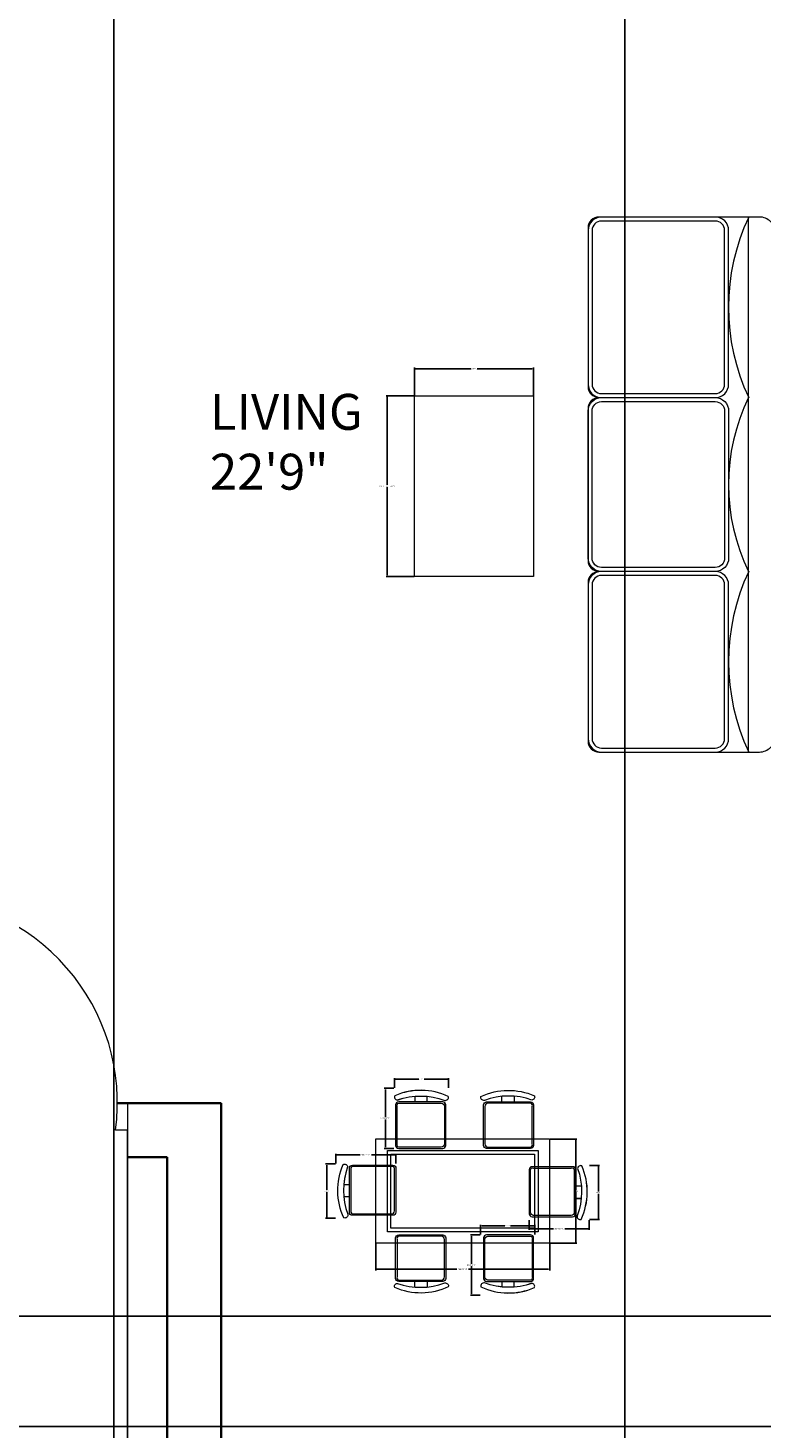
# Model space of a CAD drawing. Units: inches. Extents: x 1854 to 2495, y 1460 to 2772.
# Tile 9 of 12: x 2117 to 2239, y 1958 to 2192. Entities that reach past the tile are written whole.
import ezdxf

# ---------------------------------------------------------------- set-up
doc = ezdxf.new("R2010")
doc.units = ezdxf.units.IN
for name, color, linetype, lineweight in [('A-ANNO-DIMS', 2, 'Continuous', 18), ('A-AREA-IDEN', 7, 'Continuous', 18), ('A-DOOR', 3, 'Continuous', 18), ('A-FURN', 8, 'Continuous', 13), ('A-WALL', 7, 'Continuous', 35)]:
    doc.layers.add(name, color=color, linetype=linetype, lineweight=lineweight)
doc.styles.get("Standard").update_dxf_attribs({"font": 'arial.ttf'})
doc.dimstyles.get("Standard").update_dxf_attribs({"dimtxt": 0.18, "dimasz": 0.18, "dimexe": 0.18, "dimexo": 0.0625, "dimgap": 0.09, "dimtad": 0, "dimtih": 1, "dimtoh": 1, "dimdec": 4, "dimzin": 0, "dimdsep": 46, "dimtxsty": 'Standard', "dimcen": 0.09, "dimadec": 0, "dimazin": 0, "dimtfac": 1, "dimtdec": 4, "dimtofl": 0, "dimtmove": 0, "dimatfit": 3, "dimfxl": 1, "dimtolj": 1, "dimtzin": 0, "dimarcsym": 0})

# ---------------------------------------------------------------- blocks, each defined once
blk = doc.blocks.new('TABLE-COFFEE')
blk.add_lwpolyline([(0, 30.16), (19.85, 30.16), (19.85, 0), (0, 0)], close=True)
blk = doc.blocks.new('DINING-TABLE')
for points in [[(0, 17.41), (29.01, 17.41), (29.01, 0), (0, 0)], [(0, 17.41), (29.01, 17.41), (29.01, 0), (0, 0)], [(1.93, 15.47), (27.08, 15.47), (27.08, 1.93), (1.93, 1.93)], [(1.93, 15.47), (27.08, 15.47), (27.08, 1.93), (1.93, 1.93)], [(2.51, 14.89), (26.5, 14.89), (26.5, 2.51), (2.51, 2.51)], [(2.51, 14.89), (26.5, 14.89), (26.5, 2.51), (2.51, 2.51)]]:
    blk.add_lwpolyline(points, close=True)
blk = doc.blocks.new('DINING-CHAIR-END')
for points in [[(1.68, 0.62, -0.578392), (1.02, 0.02, -0.214524), (0.9, 8.94, -0.552014), (1.62, 8.53, 0.175809), (1.68, 0.62)], [(1.68, 0.62, -0.578392), (1.02, 0.02, -0.214524), (0.9, 8.94, -0.552014), (1.62, 8.52, 0.175809), (1.68, 0.62)], [(1.93, 8.29, -0.414214), (2.45, 8.81), (9.19, 8.81, -0.414214), (9.7, 8.29), (9.7, 0.96, -0.414214), (9.19, 0.45), (2.45, 0.45, -0.414214), (1.93, 0.96), (1.93, 8.29)], [(1.93, 8.29, -0.414214), (2.45, 8.81), (9.19, 8.81, -0.414214), (9.7, 8.29), (9.7, 0.96, -0.414214), (9.19, 0.45), (2.45, 0.45, -0.414214), (1.93, 0.96), (1.93, 8.29)], [(1.93, 3.54), (1, 3.54, 0.064759)], [(1.93, 3.54), (1, 3.54, 0.064759)]]:
    blk.add_lwpolyline(points, format="xyb")
blk.add_lwpolyline([(2.16, 8.29), (2.16, 1.19, 0.414214), (2.68, 0.68), (8.96, 0.68, 0.414214), (9.47, 1.19), (9.47, 8.29, 0.512069), (8.96, 8.58), (2.68, 8.58, 0.512069)], format="xyb", close=True)
blk.add_lwpolyline([(2.16, 8.29), (2.16, 1.19, 0.414214), (2.68, 0.68), (8.96, 0.68, 0.414214), (9.47, 1.19), (9.47, 8.29, 0.512069), (8.96, 8.58), (2.68, 8.58, 0.512069)], format="xyb", close=True)
blk.add_lwpolyline([(0.99, 5.59), (1.93, 5.59)])
blk.add_lwpolyline([(0.99, 5.59), (1.93, 5.59)])
blk = doc.blocks.new('DINING-CHAIR-01')
for points in [[(0.47, 8.09, -0.175809), (8.38, 8.03, 0.578392), (8.98, 8.69, 0.214524), (0.06, 8.81, 0.552014), (0.47, 8.09, -0.065079)], [(8.04, 7.77), (0.71, 7.77, 0.414214), (0.19, 7.26), (0.19, 0.51, 0.414214), (0.71, 0), (8.04, 0, 0.414214), (8.55, 0.51), (8.55, 7.26, 0.414214), (8.04, 7.77)], [(5.46, 7.77), (5.46, 8.7, -0.064759)]]:
    blk.add_lwpolyline(points, format="xyb")
blk.add_lwpolyline([(0.71, 7.54), (7.81, 7.54, -0.414214), (8.32, 7.03), (8.32, 0.74, -0.414214), (7.81, 0.23), (0.71, 0.23, -0.512069), (0.42, 0.74), (0.42, 7.03, -0.512069)], format="xyb", close=True)
blk.add_lwpolyline([(3.41, 8.72), (3.41, 7.77)])
blk = doc.blocks.new('DINING-CHAIR-04')
for points in [[(7.77, 8.29, 0.414214), (7.26, 8.81), (0.51, 8.81, 0.414214), (0, 8.29), (0, 0.96, 0.414214), (0.51, 0.44), (7.26, 0.44, 0.414214), (7.77, 0.96), (7.77, 8.29)], [(8.09, 8.52, -0.175809), (8.03, 0.62, 0.578392), (8.69, 0.02, 0.214524), (8.81, 8.94, 0.552014), (8.09, 8.52, -0.065079)], [(7.77, 3.53), (8.7, 3.53, -0.064759)]]:
    blk.add_lwpolyline(points, format="xyb")
blk.add_lwpolyline([(7.54, 8.29), (7.54, 1.19, -0.414214), (7.03, 0.68), (0.74, 0.68, -0.414214), (0.23, 1.19), (0.23, 8.29, -0.512069), (0.74, 8.58), (7.03, 8.58, -0.512069)], format="xyb", close=True)
blk.add_lwpolyline([(8.72, 5.59), (7.77, 5.59)])
blk = doc.blocks.new('DINING-CHAIR-06')
for points in [[(8.29, 1.93, 0.414214), (8.81, 2.45), (8.81, 9.19, 0.414214), (8.29, 9.7), (0.96, 9.7, 0.414214), (0.44, 9.19), (0.44, 2.45, 0.414214), (0.96, 1.93), (8.29, 1.93)], [(8.52, 1.62, -0.175809), (0.62, 1.68, 0.578392), (0.02, 1.02, 0.214524), (8.94, 0.9, 0.552014), (8.52, 1.62, -0.065079)], [(3.53, 1.93), (3.53, 1, -0.064759)]]:
    blk.add_lwpolyline(points, format="xyb")
blk.add_lwpolyline([(8.29, 2.16), (1.19, 2.16, -0.414214), (0.68, 2.68), (0.68, 8.96, -0.414214), (1.19, 9.47), (8.29, 9.47, -0.512069), (8.58, 8.96), (8.58, 2.68, -0.512069)], format="xyb", close=True)
blk.add_lwpolyline([(5.59, 0.99), (5.59, 1.93)])
blk = doc.blocks.new('SOFA-3-SEAT')
for points in [[(2.23, 59.19), (21.22, 59.19, 0.414214), (23.45, 61.43), (23.45, 87.12, 0.414214), (21.22, 89.35), (2.23, 89.35, 0.414214), (0, 87.12), (0, 61.43, 0.414214)], [(2.23, 59.19), (21.22, 59.19, -0.414214), (23.45, 56.96), (23.45, 32.39, -0.414214), (21.22, 30.16), (2.23, 30.16, -0.414214), (0, 32.39), (0, 56.96, -0.414214)], [(2.23, 0), (21.22, 0, 0.414214), (23.45, 2.23), (23.45, 27.92, 0.414214), (21.22, 30.16), (2.23, 30.16, 0.414214), (0, 27.92), (0, 2.23, 0.414214)]]:
    blk.add_lwpolyline(points, format="xyb", close=True)
at = {"ltscale": 0.03}
blk.add_lwpolyline([(0, 28.35), (0, 1.79, 0.414214), (1.79, 0), (28.59, 0, 0.414214), (31.27, 2.68), (31.27, 86.67, 0.414214), (28.59, 89.35), (1.79, 89.35, 0.414214), (0, 87.56), (0, 61, 0.414214), (1.79, 59.22, -1), (1.79, 59.17, 0.414214), (0, 57.38), (0, 31.96, 0.414214), (1.79, 30.18, -1), (1.79, 30.13, 0.414214)], format="xyb", close=True, dxfattribs=at)
blk.add_lwpolyline([(26.8, 0), (26.8, 89.35)])
for centre, radius, start, end in [((58.64, 74.27), 35.22, 154.6538, 205.3462), ((56.4, 44.67), 32.97, 153.869, 206.131), ((59.01, 15.08), 35.56, 154.9106, 205.0894)]:
    blk.add_arc(centre, radius, start, end)
blk = doc.blocks.new('*D23')
at = {"layer": 'A-ANNO-DIMS', "color": 0, "lineweight": -2, "transparency": 16777216}
for p, q in [((2181.17, 2130.19), (2176.52, 2130.19)), ((2176.7, 2130.01), (2176.7, 2115.3)), ((2176.7, 2100.21), (2176.7, 2114.93)), ((2181.17, 2100.03), (2176.52, 2100.03))]:
    blk.add_line(p, q, dxfattribs=at)
at = {"layer": 'A-ANNO-DIMS', "color": 0, "transparency": 16777216}
for points in [[(2176.67, 2130.01), (2176.73, 2130.01), (2176.7, 2130.19)], [(2176.67, 2100.21), (2176.73, 2100.21), (2176.7, 2100.03)]]:
    blk.add_solid(points, dxfattribs=at)
at = {"layer": 'Defpoints', "color": 0, "transparency": 16777216}
for p in [(2176.7, 2130.19), (2181.23, 2130.19), (2181.23, 2100.03)]:
    blk.add_point(p, dxfattribs=at)
at = {"layer": 'A-ANNO-DIMS', "color": 0, "transparency": 16777216, "insert": (2176.7, 2115.11), "char_height": 0.18, "attachment_point": 5}
blk.add_mtext('\\A1;COFFEE TABLE 30 TYP.', dxfattribs=at)
blk = doc.blocks.new('*D24')
at = {"layer": 'A-ANNO-DIMS', "color": 0, "lineweight": -2, "transparency": 16777216}
for p, q in [((2181.23, 2130.26), (2181.23, 2134.9)), ((2181.41, 2134.72), (2190.62, 2134.72)), ((2200.9, 2134.72), (2191.68, 2134.72)), ((2201.08, 2130.26), (2201.08, 2134.9))]:
    blk.add_line(p, q, dxfattribs=at)
at = {"layer": 'A-ANNO-DIMS', "color": 0, "transparency": 16777216}
for points in [[(2181.41, 2134.75), (2181.41, 2134.69), (2181.23, 2134.72)], [(2200.9, 2134.75), (2200.9, 2134.69), (2201.08, 2134.72)]]:
    blk.add_solid(points, dxfattribs=at)
at = {"layer": 'Defpoints', "color": 0, "transparency": 16777216}
for p in [(2201.08, 2134.72), (2181.23, 2130.19), (2201.08, 2130.19)]:
    blk.add_point(p, dxfattribs=at)
at = {"layer": 'A-ANNO-DIMS', "color": 0, "transparency": 16777216, "insert": (2191.15, 2134.72), "char_height": 0.18, "attachment_point": 5}
blk.add_mtext('\\A1;20 TYP.', dxfattribs=at)
blk = doc.blocks.new('*D33')
at = {"layer": 'A-ANNO-DIMS', "color": 0, "lineweight": -2, "transparency": 16777216}
for p, q in [((2174.78, 1988.6), (2174.78, 1984.13)), ((2203.8, 1988.6), (2203.8, 1984.13)), ((2174.96, 1984.31), (2188.33, 1984.31)), ((2203.62, 1984.31), (2190.25, 1984.31))]:
    blk.add_line(p, q, dxfattribs=at)
at = {"layer": 'A-ANNO-DIMS', "color": 0, "transparency": 16777216}
for points in [[(2174.96, 1984.34), (2174.96, 1984.28), (2174.78, 1984.31)], [(2203.62, 1984.34), (2203.62, 1984.28), (2203.8, 1984.31)]]:
    blk.add_solid(points, dxfattribs=at)
at = {"layer": 'Defpoints', "color": 0, "transparency": 16777216}
for p in [(2174.78, 1988.66), (2203.8, 1988.66), (2203.8, 1984.31)]:
    blk.add_point(p, dxfattribs=at)
at = {"layer": 'A-ANNO-DIMS', "color": 0, "transparency": 16777216, "insert": (2189.29, 1984.31), "char_height": 0.18, "attachment_point": 5}
blk.add_mtext('\\A1;TABLE 29 TYP.', dxfattribs=at)
blk = doc.blocks.new('*D34')
at = {"layer": 'A-ANNO-DIMS', "color": 0, "lineweight": -2, "transparency": 16777216}
for p, q in [((2203.86, 2006.07), (2208.33, 2006.07)), ((2208.15, 2005.89), (2208.15, 1997.55)), ((2208.15, 1988.84), (2208.15, 1997.19)), ((2203.86, 1988.66), (2208.33, 1988.66))]:
    blk.add_line(p, q, dxfattribs=at)
at = {"layer": 'A-ANNO-DIMS', "color": 0, "transparency": 16777216}
for points in [[(2208.12, 2005.89), (2208.18, 2005.89), (2208.15, 2006.07)], [(2208.12, 1988.84), (2208.18, 1988.84), (2208.15, 1988.66)]]:
    blk.add_solid(points, dxfattribs=at)
at = {"layer": 'Defpoints', "color": 0, "transparency": 16777216}
for p in [(2203.8, 2006.07), (2208.15, 2006.07), (2203.8, 1988.66)]:
    blk.add_point(p, dxfattribs=at)
at = {"layer": 'A-ANNO-DIMS', "color": 0, "transparency": 16777216, "insert": (2208.15, 1997.37), "char_height": 0.18, "attachment_point": 5}
blk.add_mtext('\\A1;17 TYP.', dxfattribs=at)
blk = doc.blocks.new('*D39')
at = {"layer": 'A-ANNO-DIMS', "color": 0, "lineweight": -2, "transparency": 16777216}
for p, q in [((2168.09, 2001.96), (2168.09, 2003.59)), ((2168.27, 2003.41), (2172.17, 2003.41)), ((2177.95, 2003.41), (2174.06, 2003.41)), ((2178.13, 2001.96), (2178.13, 2003.59))]:
    blk.add_line(p, q, dxfattribs=at)
at = {"layer": 'A-ANNO-DIMS', "color": 0, "transparency": 16777216}
for points in [[(2168.27, 2003.44), (2168.27, 2003.38), (2168.09, 2003.41)], [(2177.95, 2003.44), (2177.95, 2003.38), (2178.13, 2003.41)]]:
    blk.add_solid(points, dxfattribs=at)
at = {"layer": 'Defpoints', "color": 0, "transparency": 16777216}
for p in [(2168.09, 2001.9), (2178.13, 2003.41), (2178.13, 2001.9)]:
    blk.add_point(p, dxfattribs=at)
at = {"layer": 'A-ANNO-DIMS', "color": 0, "transparency": 16777216, "insert": (2173.11, 2003.41), "char_height": 0.18, "attachment_point": 5}
blk.add_mtext('\\A1;END A 10 TYP.', dxfattribs=at)
blk = doc.blocks.new('*D40')
at = {"layer": 'A-ANNO-DIMS', "color": 0, "lineweight": -2, "transparency": 16777216}
for p, q in [((2168.03, 2001.9), (2166.4, 2001.9)), ((2166.58, 2001.72), (2166.58, 1997.56)), ((2166.58, 1993.03), (2166.58, 1997.19)), ((2168.03, 1992.85), (2166.4, 1992.85))]:
    blk.add_line(p, q, dxfattribs=at)
at = {"layer": 'A-ANNO-DIMS', "color": 0, "transparency": 16777216}
for points in [[(2166.55, 2001.72), (2166.61, 2001.72), (2166.58, 2001.9)], [(2166.55, 1993.03), (2166.61, 1993.03), (2166.58, 1992.85)]]:
    blk.add_solid(points, dxfattribs=at)
at = {"layer": 'Defpoints', "color": 0, "transparency": 16777216}
for p in [(2166.58, 2001.9), (2168.09, 2001.9), (2168.09, 1992.85)]:
    blk.add_point(p, dxfattribs=at)
at = {"layer": 'A-ANNO-DIMS', "color": 0, "transparency": 16777216, "insert": (2166.58, 1997.37), "char_height": 0.18, "attachment_point": 5}
blk.add_mtext('\\A1;9 TYP.', dxfattribs=at)
blk = doc.blocks.new('*D41')
at = {"layer": 'A-ANNO-DIMS', "color": 0, "lineweight": -2, "transparency": 16777216}
for p, q in [((2177.81, 2014.54), (2176.19, 2014.54)), ((2176.37, 2014.36), (2176.37, 2009.7)), ((2176.37, 2004.68), (2176.37, 2009.33)), ((2177.81, 2004.5), (2176.19, 2004.5))]:
    blk.add_line(p, q, dxfattribs=at)
at = {"layer": 'A-ANNO-DIMS', "color": 0, "transparency": 16777216}
for points in [[(2176.34, 2014.36), (2176.4, 2014.36), (2176.37, 2014.54)], [(2176.34, 2004.68), (2176.4, 2004.68), (2176.37, 2004.5)]]:
    blk.add_solid(points, dxfattribs=at)
at = {"layer": 'Defpoints', "color": 0, "transparency": 16777216}
for p in [(2176.37, 2014.54), (2177.88, 2014.54), (2177.88, 2004.5)]:
    blk.add_point(p, dxfattribs=at)
at = {"layer": 'A-ANNO-DIMS', "color": 0, "transparency": 16777216, "insert": (2176.37, 2009.52), "char_height": 0.18, "attachment_point": 5}
blk.add_mtext('\\A1;SIDE A 10 TYP.', dxfattribs=at)
blk = doc.blocks.new('*D42')
at = {"layer": 'A-ANNO-DIMS', "color": 0, "lineweight": -2, "transparency": 16777216}
for p, q in [((2177.88, 2014.6), (2177.88, 2016.23)), ((2178.06, 2016.05), (2181.94, 2016.05)), ((2186.75, 2016.05), (2182.86, 2016.05)), ((2186.93, 2014.6), (2186.93, 2016.23))]:
    blk.add_line(p, q, dxfattribs=at)
at = {"layer": 'A-ANNO-DIMS', "color": 0, "transparency": 16777216}
for points in [[(2178.06, 2016.08), (2178.06, 2016.02), (2177.88, 2016.05)], [(2186.75, 2016.08), (2186.75, 2016.02), (2186.93, 2016.05)]]:
    blk.add_solid(points, dxfattribs=at)
at = {"layer": 'Defpoints', "color": 0, "transparency": 16777216}
for p in [(2186.93, 2016.05), (2177.88, 2014.54), (2186.93, 2014.54)]:
    blk.add_point(p, dxfattribs=at)
at = {"layer": 'A-ANNO-DIMS', "color": 0, "transparency": 16777216, "insert": (2182.4, 2016.05), "char_height": 0.18, "attachment_point": 5}
blk.add_mtext('\\A1;9 TYP.', dxfattribs=at)
blk = doc.blocks.new('*D43')
at = {"layer": 'A-ANNO-DIMS', "color": 0, "lineweight": -2, "transparency": 16777216}
for p, q in [((2200.37, 1992.53), (2200.37, 1990.91)), ((2210.41, 1992.53), (2210.41, 1990.91)), ((2200.55, 1991.09), (2204.45, 1991.09)), ((2210.23, 1991.09), (2206.33, 1991.09))]:
    blk.add_line(p, q, dxfattribs=at)
at = {"layer": 'A-ANNO-DIMS', "color": 0, "transparency": 16777216}
for points in [[(2200.55, 1991.12), (2200.55, 1991.06), (2200.37, 1991.09)], [(2210.23, 1991.12), (2210.23, 1991.06), (2210.41, 1991.09)]]:
    blk.add_solid(points, dxfattribs=at)
at = {"layer": 'Defpoints', "color": 0, "transparency": 16777216}
for p in [(2200.37, 1992.6), (2210.41, 1992.6), (2210.41, 1991.09)]:
    blk.add_point(p, dxfattribs=at)
at = {"layer": 'A-ANNO-DIMS', "color": 0, "transparency": 16777216, "insert": (2205.39, 1991.09), "char_height": 0.18, "attachment_point": 5}
blk.add_mtext('\\A1;END B 10 TYP.', dxfattribs=at)
blk = doc.blocks.new('*D44')
at = {"layer": 'A-ANNO-DIMS', "color": 0, "lineweight": -2, "transparency": 16777216}
for p, q in [((2210.47, 2001.65), (2212.1, 2001.65)), ((2211.92, 2001.47), (2211.92, 1997.31)), ((2211.92, 1992.78), (2211.92, 1996.94)), ((2210.47, 1992.6), (2212.1, 1992.6))]:
    blk.add_line(p, q, dxfattribs=at)
at = {"layer": 'A-ANNO-DIMS', "color": 0, "transparency": 16777216}
for points in [[(2211.89, 2001.47), (2211.95, 2001.47), (2211.92, 2001.65)], [(2211.89, 1992.78), (2211.95, 1992.78), (2211.92, 1992.6)]]:
    blk.add_solid(points, dxfattribs=at)
at = {"layer": 'Defpoints', "color": 0, "transparency": 16777216}
for p in [(2210.41, 2001.65), (2211.92, 2001.65), (2210.41, 1992.6)]:
    blk.add_point(p, dxfattribs=at)
at = {"layer": 'A-ANNO-DIMS', "color": 0, "transparency": 16777216, "insert": (2211.92, 1997.12), "char_height": 0.18, "attachment_point": 5}
blk.add_mtext('\\A1;9 TYP.', dxfattribs=at)
blk = doc.blocks.new('*D45')
at = {"layer": 'A-ANNO-DIMS', "color": 0, "lineweight": -2, "transparency": 16777216}
for p, q in [((2192.21, 1990.05), (2190.59, 1990.05)), ((2190.77, 1989.87), (2190.77, 1985.22)), ((2190.77, 1980.19), (2190.77, 1984.85)), ((2192.21, 1980.01), (2190.59, 1980.01))]:
    blk.add_line(p, q, dxfattribs=at)
at = {"layer": 'A-ANNO-DIMS', "color": 0, "transparency": 16777216}
for points in [[(2190.74, 1989.87), (2190.8, 1989.87), (2190.77, 1990.05)], [(2190.74, 1980.19), (2190.8, 1980.19), (2190.77, 1980.01)]]:
    blk.add_solid(points, dxfattribs=at)
at = {"layer": 'Defpoints', "color": 0, "transparency": 16777216}
for p in [(2190.77, 1990.05), (2192.27, 1990.05), (2192.27, 1980.01)]:
    blk.add_point(p, dxfattribs=at)
at = {"layer": 'A-ANNO-DIMS', "color": 0, "transparency": 16777216, "insert": (2190.77, 1985.03), "char_height": 0.18, "attachment_point": 5}
blk.add_mtext('\\A1;SIDE B 10 TYP.', dxfattribs=at)
blk = doc.blocks.new('*D46')
at = {"layer": 'A-ANNO-DIMS', "color": 0, "lineweight": -2, "transparency": 16777216}
for p, q in [((2192.27, 1990.12), (2192.27, 1991.74)), ((2192.45, 1991.56), (2196.34, 1991.56)), ((2201.15, 1991.56), (2197.26, 1991.56)), ((2201.33, 1990.12), (2201.33, 1991.74))]:
    blk.add_line(p, q, dxfattribs=at)
at = {"layer": 'A-ANNO-DIMS', "color": 0, "transparency": 16777216}
for points in [[(2192.45, 1991.59), (2192.45, 1991.53), (2192.27, 1991.56)], [(2201.15, 1991.59), (2201.15, 1991.53), (2201.33, 1991.56)]]:
    blk.add_solid(points, dxfattribs=at)
at = {"layer": 'Defpoints', "color": 0, "transparency": 16777216}
for p in [(2192.27, 1990.05), (2201.33, 1991.56), (2201.33, 1990.05)]:
    blk.add_point(p, dxfattribs=at)
at = {"layer": 'A-ANNO-DIMS', "color": 0, "transparency": 16777216, "insert": (2196.8, 1991.56), "char_height": 0.18, "attachment_point": 5}
blk.add_mtext('\\A1;9 TYP.', dxfattribs=at)
blk = doc.blocks.new('*D50')
at = {"layer": 'A-ANNO-DIMS', "color": 0, "lineweight": -2, "transparency": 16777216}
for p, q in [((2381.04, 2272.04), (2418.21, 2272.04)), ((2418.03, 2271.86), (2418.03, 1933.48)), ((2418.03, 1594.72), (2418.03, 1933.11)), ((2119.04, 1594.54), (2418.21, 1594.54))]:
    blk.add_line(p, q, dxfattribs=at)
at = {"layer": 'A-ANNO-DIMS', "color": 0, "transparency": 16777216}
for points in [[(2418, 2271.86), (2418.06, 2271.86), (2418.03, 2272.04)], [(2418, 1594.72), (2418.06, 1594.72), (2418.03, 1594.54)]]:
    blk.add_solid(points, dxfattribs=at)
at = {"layer": 'Defpoints', "color": 0, "transparency": 16777216}
for p in [(2380.98, 2272.04), (2418.03, 2272.04), (2118.98, 1594.54)]:
    blk.add_point(p, dxfattribs=at)
at = {"layer": 'A-ANNO-DIMS', "color": 0, "transparency": 16777216, "insert": (2418.03, 1933.29), "char_height": 0.18, "attachment_point": 5}
blk.add_mtext('\\A1;677.5', dxfattribs=at)
blk = doc.blocks.new('*D62')
at = {"layer": 'A-ANNO-DIMS', "color": 0, "lineweight": -2, "transparency": 16777216}
for p, q in [((2139.98, 2002.98), (2139.98, 1503.44)), ((2094.98, 1963.98), (2094.98, 1503.44)), ((2095.16, 1503.62), (2117.26, 1503.62)), ((2139.8, 1503.62), (2117.71, 1503.62))]:
    blk.add_line(p, q, dxfattribs=at)
at = {"layer": 'A-ANNO-DIMS', "color": 0, "transparency": 16777216}
for points in [[(2095.16, 1503.65), (2095.16, 1503.59), (2094.98, 1503.62)], [(2139.8, 1503.65), (2139.8, 1503.59), (2139.98, 1503.62)]]:
    blk.add_solid(points, dxfattribs=at)
at = {"layer": 'Defpoints', "color": 0, "transparency": 16777216}
for p in [(2139.98, 2003.04), (2094.98, 1964.04), (2139.98, 1503.62)]:
    blk.add_point(p, dxfattribs=at)
at = {"layer": 'A-ANNO-DIMS', "color": 0, "transparency": 16777216, "insert": (2117.48, 1503.62), "char_height": 0.18, "attachment_point": 5}
blk.add_mtext('\\A1;45', dxfattribs=at)
blk = doc.blocks.new('*D68')
at = {"layer": 'A-ANNO-DIMS', "color": 0, "lineweight": -2, "transparency": 16777216}
for p, q in [((2371.92, 1976.49), (1940.75, 1976.49)), ((1940.93, 1976.31), (1940.93, 1967.45)), ((1940.93, 1958.22), (1940.93, 1967.08)), ((2371.92, 1958.04), (1940.75, 1958.04))]:
    blk.add_line(p, q, dxfattribs=at)
at = {"layer": 'A-ANNO-DIMS', "color": 0, "transparency": 16777216}
for points in [[(1940.9, 1976.31), (1940.96, 1976.31), (1940.93, 1976.49)], [(1940.9, 1958.22), (1940.96, 1958.22), (1940.93, 1958.04)]]:
    blk.add_solid(points, dxfattribs=at)
at = {"layer": 'Defpoints', "color": 0, "transparency": 16777216}
for p in [(2371.98, 1976.49), (1940.93, 1958.04), (2371.98, 1958.04)]:
    blk.add_point(p, dxfattribs=at)
at = {"layer": 'A-ANNO-DIMS', "color": 0, "transparency": 16777216, "insert": (1940.93, 1967.27), "char_height": 0.18, "attachment_point": 5}
blk.add_mtext('\\A1;18.442', dxfattribs=at)
blk = doc.blocks.new('*D71')
at = {"layer": 'A-ANNO-DIMS', "color": 0, "lineweight": -2, "transparency": 16777216}
for p, q in [((2095.37, 2002.98), (2095.37, 1503.44)), ((2133.34, 2002.98), (2133.34, 1503.44)), ((2095.55, 1503.62), (2113.96, 1503.62)), ((2133.16, 1503.62), (2114.75, 1503.62))]:
    blk.add_line(p, q, dxfattribs=at)
at = {"layer": 'A-ANNO-DIMS', "color": 0, "transparency": 16777216}
for points in [[(2095.55, 1503.65), (2095.55, 1503.59), (2095.37, 1503.62)], [(2133.16, 1503.65), (2133.16, 1503.59), (2133.34, 1503.62)]]:
    blk.add_solid(points, dxfattribs=at)
at = {"layer": 'Defpoints', "color": 0, "transparency": 16777216}
for p in [(2095.37, 2003.04), (2133.34, 2003.04), (2133.34, 1503.62)]:
    blk.add_point(p, dxfattribs=at)
at = {"layer": 'A-ANNO-DIMS', "color": 0, "transparency": 16777216, "insert": (2114.36, 1503.62), "char_height": 0.18, "attachment_point": 5}
blk.add_mtext('\\A1;37.97', dxfattribs=at)
blk = doc.blocks.new('*D73')
at = {"layer": 'A-ANNO-DIMS', "color": 0, "lineweight": -2, "transparency": 16777216}
for p, q in [((2131.08, 2220.98), (2131.08, 1503.44)), ((2216.32, 2220.98), (2216.32, 1503.44)), ((2131.26, 1503.62), (2173.31, 1503.62)), ((2216.14, 1503.62), (2174.1, 1503.62))]:
    blk.add_line(p, q, dxfattribs=at)
at = {"layer": 'A-ANNO-DIMS', "color": 0, "transparency": 16777216}
for points in [[(2131.26, 1503.65), (2131.26, 1503.59), (2131.08, 1503.62)], [(2216.14, 1503.65), (2216.14, 1503.59), (2216.32, 1503.62)]]:
    blk.add_solid(points, dxfattribs=at)
at = {"layer": 'Defpoints', "color": 0, "transparency": 16777216}
for p in [(2131.08, 2221.04), (2216.32, 2221.04), (2216.32, 1503.62)]:
    blk.add_point(p, dxfattribs=at)
at = {"layer": 'A-ANNO-DIMS', "color": 0, "transparency": 16777216, "insert": (2173.7, 1503.62), "char_height": 0.18, "attachment_point": 5}
blk.add_mtext('\\A1;85.25', dxfattribs=at)

msp = doc.modelspace()

# ---------------------------------------------------------------- linework, layer by layer
at = {"layer": 'A-DOOR'}
for p, q in [((2133.341, 2012.0449), (2133.341, 2003.0449)), ((2133.341, 2007.5449), (2131.341, 2007.5449)), ((2133.341, 2003.0449), (2133.341, 2007.5449))]:
    msp.add_line(p, q, dxfattribs=at)
msp.add_arc((2097.3698, 2012.1239), 34.2784, 352.32339, 90, dxfattribs=at)
at = {"layer": 'A-FURN'}
for points in [[(2212.444, 2130.5637), (2231.4306, 2130.5637, 0.41421356), (2232.9942, 2132.1273), (2232.9942, 2157.8152, 0.41421356), (2231.4306, 2159.3788), (2212.444, 2159.3788, 0.41421356), (2210.8804, 2157.8152), (2210.8804, 2132.1273, 0.41421356)], [(2212.444, 2129.2235), (2231.4306, 2129.2235, -0.41421356), (2232.9942, 2127.6599), (2232.9942, 2103.0889, -0.41421356), (2231.4306, 2101.5253), (2212.444, 2101.5253, -0.41421356), (2210.8804, 2103.0889), (2210.8804, 2127.6599, -0.41421356)], [(2212.444, 2071.37), (2231.4306, 2071.37, 0.41421356), (2232.9942, 2072.9336), (2232.9942, 2098.6214, 0.41421356), (2231.4306, 2100.1851), (2212.444, 2100.1851, 0.41421356), (2210.8804, 2098.6214), (2210.8804, 2072.9336, 0.41421356)], [(2178.6067, 2012.0352), (2185.7081, 2012.0352, -0.41421356), (2186.2213, 2011.522), (2186.2213, 2005.2394, -0.41421356), (2185.7081, 2004.7262), (2178.6067, 2004.7262, -0.51206948), (2178.3216, 2005.2394), (2178.3216, 2011.522, -0.51206948)], [(2200.5945, 2012.0355), (2193.4931, 2012.0355, 0.41421356), (2192.9799, 2011.5223), (2192.9799, 2005.2397, 0.41421356), (2193.4931, 2004.7265), (2200.5945, 2004.7265, 0.51206948), (2200.8796, 2005.2397), (2200.8796, 2011.5223, 0.51206948)], [(2200.5945, 2012.0352), (2193.4932, 2012.0352, 0.41421356), (2192.9799, 2011.522), (2192.9799, 2005.2394, 0.41421356), (2193.4932, 2004.7262), (2200.5945, 2004.7262, 0.51206948), (2200.8796, 2005.2394), (2200.8796, 2011.522, 0.51206948)], [(2207.9075, 2000.9187), (2207.9075, 1993.8173, -0.41421356), (2207.3943, 1993.3041), (2201.1117, 1993.3041, -0.41421356), (2200.5985, 1993.8173), (2200.5985, 2000.9187, -0.51206948), (2201.1117, 2001.2038), (2207.3943, 2001.2038, -0.51206948)], [(2178.6067, 1982.5147), (2185.708, 1982.5147, 0.41421356), (2186.2213, 1983.0279), (2186.2213, 1989.3105, 0.41421356), (2185.708, 1989.8237), (2178.6067, 1989.8237, 0.51206948), (2178.3216, 1989.3105), (2178.3216, 1983.0279, 0.51206948)], [(2178.6067, 1982.5144), (2185.7081, 1982.5144, 0.41421356), (2186.2213, 1983.0276), (2186.2213, 1989.3102, 0.41421356), (2185.7081, 1989.8234), (2178.6067, 1989.8234, 0.51206948), (2178.3216, 1989.3102), (2178.3216, 1983.0276, 0.51206948)]]:
    msp.add_lwpolyline(points, format="xyb", close=True, dxfattribs=at)
for points in [[(2178.3728, 2012.5836, -0.17580919), (2186.2745, 2012.5237, 0.57839206), (2186.8731, 2013.1819, 0.21452438), (2177.9538, 2013.3016, 0.55201397), (2178.3728, 2012.5835, -0.06507904)], [(2183.3626, 2012.2664), (2183.3626, 2013.1941, -0.06475861)], [(2192.9267, 2012.524, -0.57839206), (2192.3281, 2013.1822, -0.21452438), (2201.2474, 2013.3019, -0.55201397), (2200.8284, 2012.5839, 0.1758092), (2192.9267, 2012.524)], [(2192.9267, 2012.5237, -0.57839206), (2192.3281, 2013.1819, -0.21452438), (2201.2475, 2013.3016, -0.55201397), (2200.8284, 2012.5835, 0.1758092), (2192.9267, 2012.5237)], [(2195.8386, 2012.2667), (2195.8386, 2013.1945, 0.06475861)], [(2195.8386, 2012.2664), (2195.8386, 2013.1941, 0.06475861)], [(2185.9393, 2012.2664), (2178.6036, 2012.2664, 0.41421356), (2178.0904, 2011.7532), (2178.0904, 2005.0082, 0.41421356), (2178.6036, 2004.495), (2185.9393, 2004.495, 0.41421356), (2186.4525, 2005.0082), (2186.4525, 2011.7532, 0.41421356), (2185.9393, 2012.2664)], [(2200.5976, 2012.2667, -0.41421356), (2201.1108, 2011.7535), (2201.1108, 2005.0085, -0.41421356), (2200.5976, 2004.4953), (2193.2619, 2004.4953, -0.41421356), (2192.7487, 2005.0085), (2192.7487, 2011.7535, -0.41421356), (2193.2619, 2012.2667), (2200.5976, 2012.2667)], [(2200.5976, 2012.2664, -0.41421356), (2201.1108, 2011.7532), (2201.1108, 2005.0082, -0.41421356), (2200.5976, 2004.495), (2193.262, 2004.495, -0.41421356), (2192.7487, 2005.0082), (2192.7487, 2011.7532, -0.41421356), (2193.262, 2012.2664), (2200.5976, 2012.2664)], [(2208.1387, 2000.9218, 0.41421356), (2207.6255, 2001.435), (2200.8805, 2001.435, 0.41421356), (2200.3673, 2000.9218), (2200.3673, 1993.5861, 0.41421356), (2200.8805, 1993.0729), (2207.6255, 1993.0729, 0.41421356), (2208.1387, 1993.5861), (2208.1387, 2000.9218)], [(2208.4558, 2001.1526, -0.17580919), (2208.396, 1993.2509, 0.57839206), (2209.0542, 1992.6523, 0.21452438), (2209.1739, 2001.5716, 0.55201397), (2208.4558, 2001.1526, -0.06507904)], [(2208.1387, 1996.1628), (2209.0664, 1996.1628, -0.06475861)], [(2185.9393, 1982.2835), (2178.6036, 1982.2835, -0.41421356), (2178.0904, 1982.7967), (2178.0904, 1989.5417, -0.41421356), (2178.6036, 1990.0549), (2185.9393, 1990.0549, -0.41421356), (2186.4525, 1989.5417), (2186.4525, 1982.7967, -0.41421356), (2185.9393, 1982.2835)], [(2185.9393, 1982.2832), (2178.6036, 1982.2832, -0.41421356), (2178.0904, 1982.7964), (2178.0904, 1989.5414, -0.41421356), (2178.6036, 1990.0546), (2185.9393, 1990.0546, -0.41421356), (2186.4525, 1989.5414), (2186.4525, 1982.7964, -0.41421356), (2185.9393, 1982.2832)], [(2186.2745, 1982.0262, -0.57839206), (2186.8731, 1981.368, -0.21452438), (2177.9538, 1981.2483, -0.55201397), (2178.3728, 1981.9664, 0.17580929), (2186.2745, 1982.0262)], [(2186.2745, 1982.0259, -0.57839206), (2186.8731, 1981.3677, -0.21452438), (2177.9538, 1981.248, -0.55201397), (2178.3728, 1981.9661, 0.17580929), (2186.2745, 1982.0259)], [(2183.3626, 1982.2835), (2183.3626, 1981.3558, 0.06475861)], [(2183.3626, 1982.2832), (2183.3626, 1981.3555, 0.06475861)]]:
    msp.add_lwpolyline(points, format="xyb", dxfattribs=at)
for points in [[(2181.3092, 2013.211), (2181.3092, 2012.2664)], [(2197.892, 2013.2113), (2197.892, 2012.2667)], [(2197.892, 2013.211), (2197.892, 2012.2664)], [(2209.0833, 1998.2162), (2208.1387, 1998.2162)], [(2181.3092, 1981.3389), (2181.3092, 1982.2835)], [(2181.3092, 1981.3386), (2181.3092, 1982.2832)]]:
    msp.add_lwpolyline(points, dxfattribs=at)
at = {"layer": 'A-WALL'}
for p, q in [((2131.6481, 2012.0449), (2139.9824, 2012.0449)), ((2139.9824, 2012.0449), (2148.9824, 2012.0449)), ((2148.9824, 2012.0449), (2148.9824, 1937.5287)), ((2133.341, 2003.0449), (2139.9824, 2003.0449)), ((2139.9824, 2003.0449), (2139.9824, 1847.0449))]:
    msp.add_line(p, q, dxfattribs=at)

# ---------------------------------------------------------------- block references
at = {"layer": 'A-FURN'}
for name, p in [('SOFA-3-SEAT', (2210.21, 2070.7)), ('TABLE-COFFEE', (2181.2294, 2100.0316)), ('DINING-CHAIR-01', (2177.898, 2004.495)), ('DINING-TABLE', (2174.784, 1988.665)), ('DINING-CHAIR-END', (2168.431, 1992.879)), ('DINING-CHAIR-04', (2200.367, 1992.629)), ('DINING-CHAIR-06', (2192.304, 1980.351))]:
    msp.add_blockref(name, p, dxfattribs=at)
at = {"layer": 'A-FURN', "rotation": 270.0000011780324}
msp.add_blockref('DINING-CHAIR-04', (2192.3045, 1990.0549), dxfattribs=at)

# ---------------------------------------------------------------- texts
at = {"layer": 'A-AREA-IDEN', "insert": (2147.0951, 2130.5139), "char_height": 6, "attachment_point": 1}
msp.add_mtext_dynamic_manual_height_columns('LIVING\\P22\'9"', width=144.246938, gutter_width=12.5, heights=[0], dxfattribs=at)

# ---------------------------------------------------------------- dimensions: what is measured, and where the dimension line sits
at = {"layer": 'A-ANNO-DIMS'}
for base, p1, p2, override, picture, middle in [((2418.0324, 2272.0449), (2118.9824, 1594.5449), (2380.9824, 2272.0449), {"dimdec": 1, "dimlfac": 1, "dimrnd": 0, "dimzin": 0, "dimdsep": 46, "dimlunit": 2}, '*D50', (2418.0324, 1933.2949)), ((1940.93239, 1958.04492), (2371.98239, 1976.48735), (2371.98239, 1958.04492), {"dimdec": 3, "dimlfac": 1, "dimrnd": 0, "dimzin": 0, "dimdsep": 46, "dimlunit": 2}, '*D68', (1940.93239, 1967.26613))]:
    dim = msp.add_linear_dim(base=base, p1=p1, p2=p2, angle=90, dimstyle='Standard', override=override, dxfattribs=at)
    dim.commit()
    dim.dimension.update_dxf_attribs({"geometry": picture, "text_midpoint": middle})
for base, p1, p2, override, picture, middle in [((2216.3239, 1503.6207), (2131.0775, 2221.0449), (2216.3239, 2221.0449), {"dimdec": 2, "dimlfac": 1, "dimrnd": 0, "dimzin": 0, "dimdsep": 46, "dimlunit": 2}, '*D73', (2173.7007, 1503.6207)), ((2139.9824, 1503.6207), (2094.9824, 1964.0449), (2139.9824, 2003.0449), {"dimdec": 0, "dimlfac": 1, "dimrnd": 0, "dimzin": 0, "dimdsep": 46, "dimlunit": 2}, '*D62', (2117.4824, 1503.6207)), ((2133.341, 1503.6207), (2095.3698, 2003.0449), (2133.341, 2003.0449), {"dimdec": 2, "dimlfac": 1, "dimrnd": 0, "dimzin": 0, "dimdsep": 46, "dimlunit": 2}, '*D71', (2114.3554, 1503.6207))]:
    dim = msp.add_linear_dim(base=base, p1=p1, p2=p2, dimstyle='Standard', override=override, dxfattribs=at)
    dim.commit()
    dim.dimension.update_dxf_attribs({"geometry": picture, "text_midpoint": middle})
for base, p1, p2, text, picture, middle in [((2201.076, 2134.7177), (2181.2289, 2130.1934), (2201.076, 2130.1934), '<> TYP.', '*D24', (2191.1525, 2134.7177)), ((2186.9293, 2016.0461), (2177.8757, 2014.5395), (2186.9293, 2014.5395), '<> TYP.', '*D42', (2182.4025, 2016.0461)), ((2178.1348, 2003.4078), (2168.0906, 2001.9012), (2178.1348, 2001.9012), 'END A <> TYP.', '*D39', (2173.1127, 2003.4078)), ((2210.4114, 1991.0898), (2200.3672, 1992.5964), (2210.4114, 1992.5964), 'END B <> TYP.', '*D43', (2205.3893, 1991.0898)), ((2201.3255, 1991.5616), (2192.2719, 1990.0549), (2201.3255, 1990.0549), '<> TYP.', '*D46', (2196.7987, 1991.5616)), ((2203.7952, 1984.3132), (2174.7845, 1988.6648), (2203.7952, 1988.6648), 'TABLE <> TYP.', '*D33', (2189.2898, 1984.3132))]:
    dim = msp.add_linear_dim(base=base, p1=p1, p2=p2, text=text, dimstyle='Standard', override={"dimdec": 0, "dimlfac": 1, "dimrnd": 0, "dimzin": 0, "dimdsep": 46, "dimlunit": 2}, dxfattribs=at)
    dim.commit()
    dim.dimension.update_dxf_attribs({"geometry": picture, "text_midpoint": middle})
for base, p1, p2, text, picture, middle in [((2176.7047, 2130.1934), (2181.2289, 2100.0318), (2181.2289, 2130.1934), 'COFFEE TABLE <> TYP.', '*D23', (2176.7047, 2115.1126)), ((2176.3691, 2014.5395), (2177.8757, 2004.4953), (2177.8757, 2014.5395), 'SIDE A <> TYP.', '*D41', (2176.3691, 2009.5174)), ((2208.1468, 2006.0716), (2203.7952, 1988.6648), (2203.7952, 2006.0716), '<> TYP.', '*D34', (2208.1468, 1997.3682)), ((2166.584, 2001.9012), (2168.0906, 1992.8474), (2168.0906, 2001.9012), '<> TYP.', '*D40', (2166.584, 1997.3743)), ((2211.9181, 2001.65), (2210.4114, 1992.5964), (2210.4114, 2001.65), '<> TYP.', '*D44', (2211.9181, 1997.1232)), ((2190.7653, 1990.0549), (2192.2719, 1980.0107), (2192.2719, 1990.0549), 'SIDE B <> TYP.', '*D45', (2190.7653, 1985.0328))]:
    dim = msp.add_linear_dim(base=base, p1=p1, p2=p2, angle=90, text=text, dimstyle='Standard', override={"dimdec": 0, "dimlfac": 1, "dimrnd": 0, "dimzin": 0, "dimdsep": 46, "dimlunit": 2}, dxfattribs=at)
    dim.commit()
    dim.dimension.update_dxf_attribs({"geometry": picture, "text_midpoint": middle})

doc.saveas('drawing.dxf')
